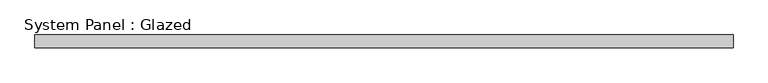
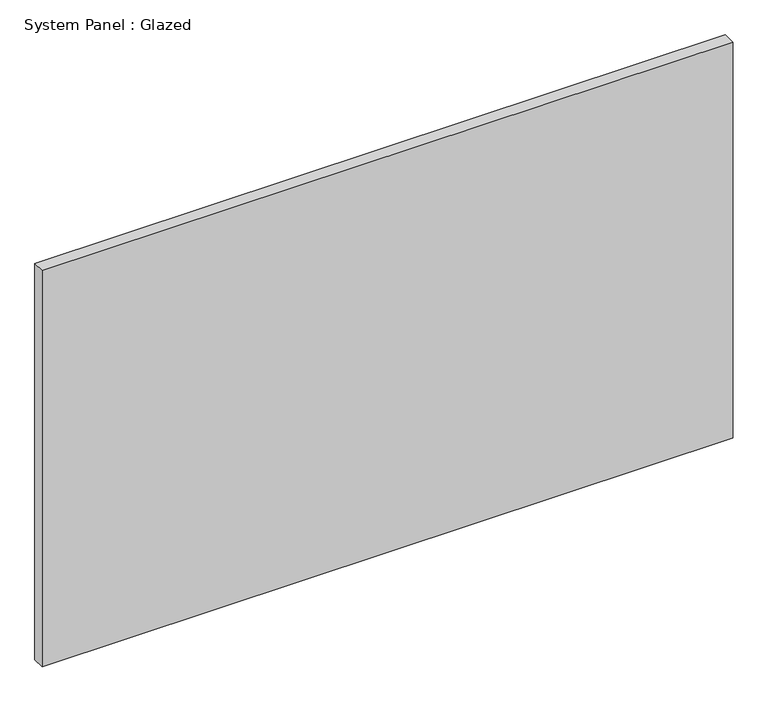
"""IFC4 building model written with IfcOpenShell, lengths in millimetres: plate geometry, System Panel : Glazed."""

from ifc_helpers import new_model, si_unit, origin, origin_with_axes, place, context, project, spatial, polyline, outline, extrude, source, transform, mapped, element, save


def system_panel_glazed_5760c905(model_context):
    return source(origin(), model_context, "Body", "SweptSolid", [
        extrude(outline(polyline([(701.6749999, -44.45), (-701.6749999, -44.45), (-701.6749999, -19.05), (701.6749999, -19.05), (701.6749999, -44.45)])), origin_with_axes(), (0.0, 0.0, 1.0), 850.9),
    ])


if __name__ == "__main__":
    model = new_model("IFC4")
    model_context = context("Model", 3, world=origin())
    ifc_project = project(units=[si_unit("LENGTHUNIT", "METRE", prefix="MILLI")], contexts=[model_context])
    site = spatial("IfcSite", under=ifc_project)
    building = spatial("IfcBuilding", under=site)
    placement = place(None, origin())
    system_panel_glazed_shape = system_panel_glazed_5760c905(model_context)
    element("IfcPlate", 1, ObjectType="System Panel : Glazed", at=placement, inside=building, context=model_context, shape_type="MappedRepresentation", body=[
        mapped(system_panel_glazed_shape, transform((0.0, 0.0, 0.0), x_axis=(1.0, 0.0, 0.0), y_axis=(0.0, 1.0, 0.0), z_axis=(0.0, 0.0, 1.0))),
    ])
    save(model, "model.ifc")

# Revit data of these elements
# Type "System Panel : Glazed"
#   Construction Type Id = "GSP4R"
#   Analytic Construction = "1/8 in Pilkington single glazing"
#   Visual Light Transmittance = 0.9
#   Solar Heat Gain Coefficient = 0.86
#   Heat Transfer Coefficient (U) = 1.18115 BTU/(h·ft²·°F)
#   Define Thermal Properties by = 1
# Element 1 (IfcPlate, "System Panel : Glazed")
#   Materials on its faces: "Glass"
# Materials
#   "Glass": class "Glass", colour RGB 0 128 192, transparency 0.75, Description = "Soda Lime Glass", Cost = 0
